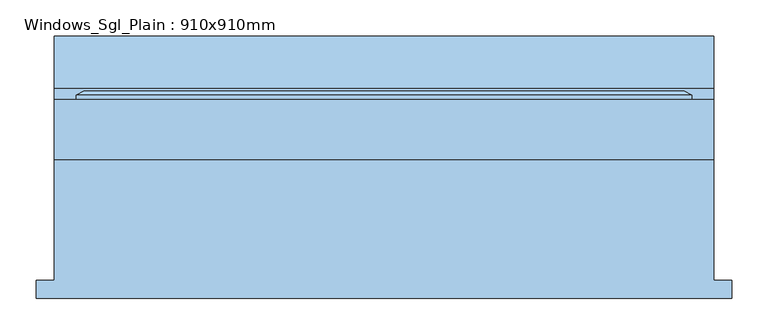
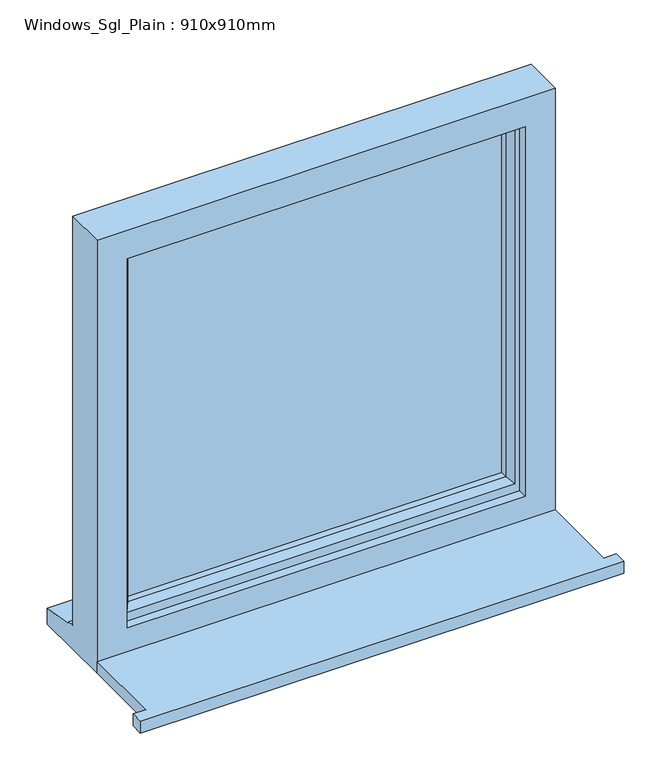
"""IFC4 building model written with IfcOpenShell, lengths in millimetres: window geometry, Windows_Sgl_Plain : 910x910mm."""

from ifc_helpers import new_model, si_unit, frame, origin, place, context, project, spatial, polyline, outline, extrude, faceted_brep, source, transform, mapped, element, save


def windows_sgl_plain_910x910mm_cb8bb1e6(model_context):
    return source(origin(), model_context, "Body", "SolidModel", [
        extrude(outline(polyline([(-480.0, -166.5434322), (-480.0, -141.5434322), (-455.0, -141.5434322), (-455.0, 25.4565678), (455.0, 25.4565678), (455.0, -141.5434322), (480.0, -141.5434322), (480.0, -166.5434322), (-480.0, -166.5434322)])), frame((0.0, 0.0, 1200.0), z_axis=(0.0, 0.0, 1.0), x_axis=(1.0, 0.0, 0.0)), (0.0, 0.0, 1.0), 25.0),
        faceted_brep([(-455.0, 25.4565678, 1200.0), (455.0, 25.4565678, 1200.0), (455.0, 25.4565678, 2110.0), (-455.0, 25.4565678, 2110.0), (-395.0, 25.4565678, 2050.0), (395.0, 25.4565678, 2050.0), (395.0, 25.4565678, 1275.0), (-395.0, 25.4565678, 1275.0), (-455.0, 108.4565678, 2110.0), (-455.0, 108.4565678, 1251.0), (-455.0, 123.4565678, 1249.68767), (-455.0, 123.4565678, 1244.7449676), (-455.0, 195.9565678, 1233.8088847), (-455.0, 195.9565678, 1200.0), (455.0, 108.4565678, 2110.0), (455.0, 108.4565678, 1251.0), (-415.0, 108.4565678, 2070.0), (-415.0, 108.4565678, 1263.0), (415.0, 108.4565678, 1263.0), (415.0, 108.4565678, 2070.0), (-415.0, 43.4565678, 2070.0), (-415.0, 43.4565678, 1263.0), (415.0, 43.4565678, 2070.0), (415.0, 43.4565678, 1263.0), (-395.0, 43.4565678, 2050.0), (-395.0, 43.4565678, 1275.0), (395.0, 43.4565678, 1275.0), (395.0, 43.4565678, 2050.0), (455.0, 195.9565678, 1200.0), (455.0, 195.9565678, 1233.8088847), (455.0, 123.4565678, 1244.7449676), (455.0, 123.4565678, 1249.68767)], [[[0, 1, 2, 3], [4, 5, 6, 7]], [[0, 3, 8, 9, 10, 11, 12, 13]], [[9, 8, 14, 15], [16, 17, 18, 19]], [[17, 16, 20, 21]], [[20, 22, 23, 21], [24, 25, 26, 27]], [[24, 4, 7, 25]], [[3, 2, 14, 8]], [[16, 19, 22, 20]], [[5, 4, 24, 27]], [[15, 14, 2, 1, 28, 29, 30, 31]], [[19, 18, 23, 22]], [[5, 27, 26, 6]], [[28, 1, 0, 13]], [[29, 28, 13, 12]], [[30, 29, 12, 11]], [[31, 30, 11, 10]], [[15, 31, 10, 9]], [[21, 23, 18, 17]], [[7, 6, 26, 25]]]),
        extrude(outline(polyline([(385.0, 72.4565678), (-385.0, 72.4565678), (-385.0, 96.4565678), (385.0, 96.4565678), (385.0, 72.4565678)])), frame((0.0, 0.0, 1293.0), z_axis=(0.0, 0.0, 1.0), x_axis=(1.0, 0.0, 0.0)), (0.0, 0.0, 1.0), 747.0),
        faceted_brep([(-425.0, 108.4565678, 2080.0), (-425.0, 114.2300705, 2080.0), (-425.0, 114.2300705, 1253.0), (-425.0, 108.4565678, 1253.0), (-415.0, 43.4565678, 2070.0), (-415.0, 108.4565678, 2070.0), (-415.0, 108.4565678, 1263.0), (-415.0, 43.4565678, 1263.0), (-375.0, 57.9494677, 2030.0), (-385.1480377, 43.4565678, 2040.1480377), (-385.1480377, 43.4565678, 1292.8519623), (-375.0, 57.9494677, 1303.0), (-375.0, 72.4565678, 2030.0), (-375.0, 72.4565678, 1303.0), (-385.0, 96.4565678, 2040.0), (-385.0, 72.4565678, 2040.0), (-385.0, 72.4565678, 1293.0), (-385.0, 96.4565678, 1293.0), (-375.0, 114.2300705, 2030.0), (-375.0, 96.4565678, 2030.0), (-375.0, 96.4565678, 1303.0), (-375.0, 114.2300705, 1303.0), (-392.4457548, 120.0035732, 2047.4457548), (-392.4457548, 120.0035732, 1285.5542452), (-414.2153903, 120.0035732, 2069.2153903), (-414.2153903, 120.0035732, 1263.7846097), (425.0, 114.2300705, 1253.0), (425.0, 108.4565678, 1253.0), (415.0, 108.4565678, 1263.0), (415.0, 43.4565678, 1263.0), (385.1480377, 43.4565678, 1292.8519623), (375.0, 57.9494677, 1303.0), (375.0, 72.4565678, 1303.0), (385.0, 72.4565678, 1293.0), (385.0, 96.4565678, 1293.0), (375.0, 96.4565678, 1303.0), (375.0, 114.2300705, 1303.0), (392.4457548, 120.0035732, 1285.5542452), (414.2153903, 120.0035732, 1263.7846097), (425.0, 114.2300705, 2080.0), (425.0, 108.4565678, 2080.0), (415.0, 108.4565678, 2070.0), (415.0, 43.4565678, 2070.0), (385.1480377, 43.4565678, 2040.1480377), (375.0, 57.9494677, 2030.0), (375.0, 72.4565678, 2030.0), (385.0, 72.4565678, 2040.0), (385.0, 96.4565678, 2040.0), (375.0, 96.4565678, 2030.0), (375.0, 114.2300705, 2030.0), (392.4457548, 120.0035732, 2047.4457548), (414.2153903, 120.0035732, 2069.2153903)], [[[0, 1, 2, 3]], [[4, 5, 6, 7]], [[8, 9, 10, 11]], [[12, 8, 11, 13]], [[14, 15, 16, 17]], [[18, 19, 20, 21]], [[22, 18, 21, 23]], [[1, 24, 25, 2]], [[3, 2, 26, 27]], [[7, 6, 28, 29]], [[11, 10, 30, 31]], [[13, 11, 31, 32]], [[17, 16, 33, 34]], [[21, 20, 35, 36]], [[23, 21, 36, 37]], [[2, 25, 38, 26]], [[27, 26, 39, 40]], [[29, 28, 41, 42]], [[31, 30, 43, 44]], [[32, 31, 44, 45]], [[34, 33, 46, 47]], [[36, 35, 48, 49]], [[37, 36, 49, 50]], [[26, 38, 51, 39]], [[40, 39, 1, 0]], [[3, 27, 40, 0], [5, 41, 28, 6]], [[42, 41, 5, 4]], [[7, 29, 42, 4], [9, 43, 30, 10]], [[44, 43, 9, 8]], [[45, 44, 8, 12]], [[15, 46, 33, 16], [13, 32, 45, 12]], [[47, 46, 15, 14]], [[17, 34, 47, 14], [19, 48, 35, 20]], [[49, 48, 19, 18]], [[50, 49, 18, 22]], [[24, 51, 38, 25], [23, 37, 50, 22]], [[39, 51, 24, 1]]]),
    ])


if __name__ == "__main__":
    model = new_model("IFC4")
    model_context = context("Model", 3, world=origin())
    ifc_project = project(units=[si_unit("LENGTHUNIT", "METRE", prefix="MILLI")], contexts=[model_context])
    site = spatial("IfcSite", under=ifc_project)
    building = spatial("IfcBuilding", under=site)
    placement = place(None, origin())
    windows_sgl_plain_910x910mm_shape = windows_sgl_plain_910x910mm_cb8bb1e6(model_context)
    element("IfcWindow", 1, ObjectType="Windows_Sgl_Plain : 910x910mm", at=placement, inside=building, context=model_context, shape_type="MappedRepresentation", body=[
        mapped(windows_sgl_plain_910x910mm_shape, transform((0.0, 0.0, 0.0), x_axis=(1.0, 0.0, 0.0), y_axis=(0.0, 1.0, 0.0), z_axis=(0.0, 0.0, 1.0))),
    ])
    save(model, "model.ifc")

# Revit data of these elements
# Type "Windows_Sgl_Plain : 910x910mm"
#   Type Mark = "44"
#   Operation = "SinglePanel"
#   Construction Type Id = "SGL"
#   Manufacturer = "Revit"
#   Keynote = "L10"
#   Analytic Construction = "Large single-glazed windows"
#   Wrap Layers (Ext) from Ext = 102.5 mm
#   Wrap Layers (Int) from Ext = 177.5 mm
#   Window Board Projection = 25 mm
#   Window Board Extension = 25 mm
#   Visual Light Transmittance = 0.9
#   Solar Heat Gain Coefficient = 0.86
#   Rough Width = 910 mm
#   Rough Height = 910 mm
#   Height = 910 mm
#   Width = 910 mm
#   Heat Transfer Coefficient (U) = 5.5617 W/(m²·K)
#   Glazing Thickness = 24 mm
#   FrameOffset - External = 50 mm
#   Frame Depth = 65 mm
#   Default Head Height = 2110 mm
#   Cill Depth = 87.5 mm
#   Cavity Closer Width = 50 mm
#   Cavity Closer Offset from Ext = 102.5 mm
#   Cavity Closer Depth = 85 mm
#   Define Thermal Properties by = 1
#   Vis - Cavity Closers = yes
#   Define Thermal Properties by = 1
#   Material Trim = Window Frame
#   Material Glass = Glass
#   Material Frame = Window Frame
#   Wall Closure = (empty or 0)
# Element 1 (IfcWindow, "Windows_Sgl_Plain : 910x910mm")
#   Materials on its faces: "Window Frame", "Glass"
# Materials
#   "Window Frame": colour RGB 249 249 249, transparency 0, Keynote = "L10", Cost = 0
#   "Glass": class "Glass", colour RGB 0 128 192, transparency 0.9, Description = "Soda Lime Glass", Cost = 0
